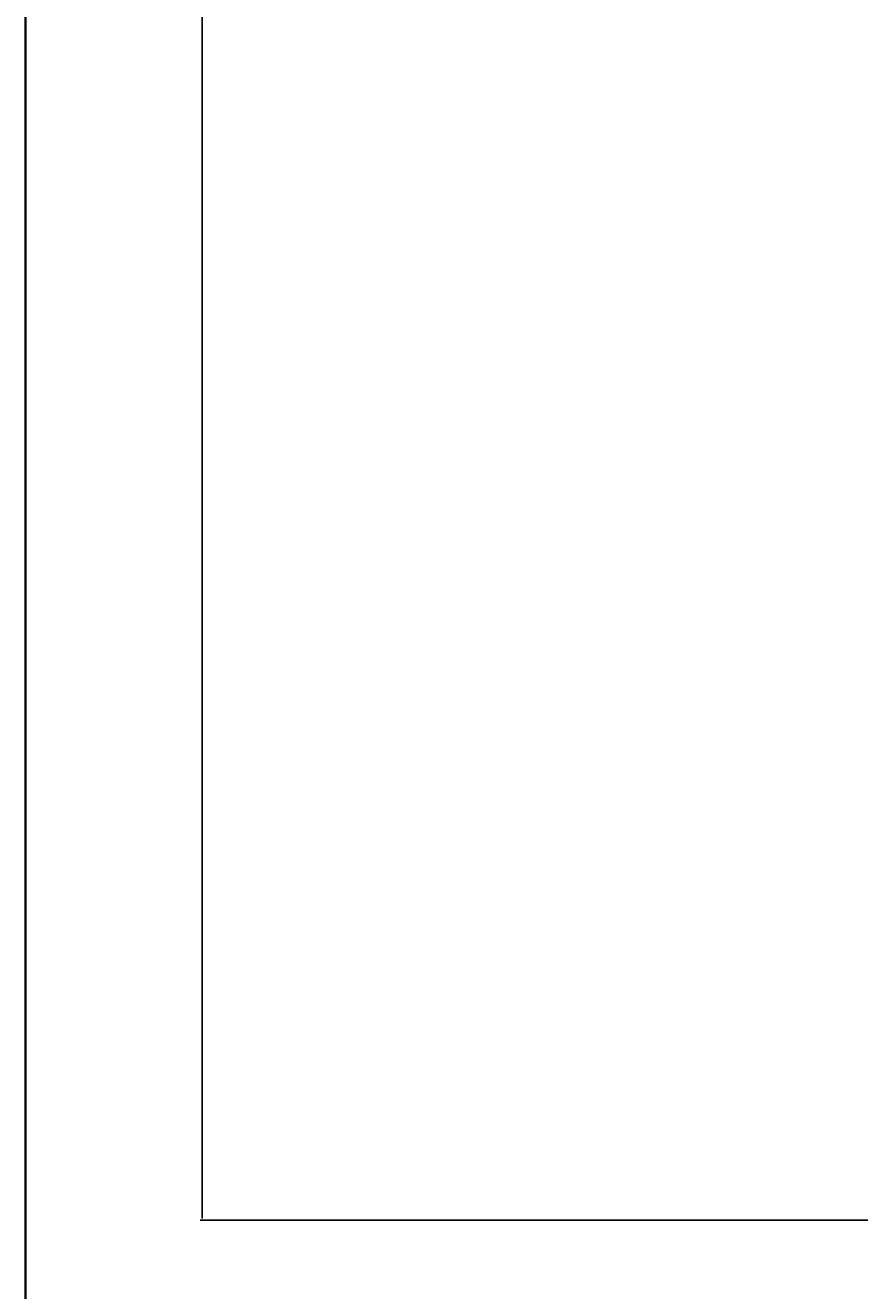
# Model space of a CAD drawing. Units: inches. Extents: x 1885 to 2748, y 783 to 2421.
# Tile 2 of 117: x 1885 to 1969, y 1050 to 1178. Entities that reach past the tile are written whole.
import ezdxf

# ---------------------------------------------------------------- set-up
doc = ezdxf.new("R2010")
doc.units = ezdxf.units.IN
doc.layers.add('A-ANNO-DIMS', color=2, linetype='Continuous', lineweight=18)
doc.layers.add('A-ANNO-TTLB', color=7, linetype='Continuous', lineweight=35)
doc.styles.get("Standard").update_dxf_attribs({"font": 'arial.ttf'})
doc.dimstyles.get("Standard").update_dxf_attribs({"dimtxt": 0.18, "dimasz": 0.18, "dimexe": 0.18, "dimexo": 0.0625, "dimgap": 0.09, "dimtad": 0, "dimtih": 1, "dimtoh": 1, "dimdec": 4, "dimzin": 0, "dimdsep": 46, "dimtxsty": 'Standard', "dimcen": 0.09, "dimadec": 0, "dimazin": 0, "dimtfac": 1, "dimtdec": 4, "dimtofl": 0, "dimtmove": 0, "dimatfit": 3, "dimfxl": 1, "dimtolj": 1, "dimtzin": 0, "dimarcsym": 0})

# ---------------------------------------------------------------- blocks, each defined once
blk = doc.blocks.new('*D45')
at = {"layer": 'A-ANNO-DIMS', "color": 0, "lineweight": -2, "transparency": 16777216}
for p, q in [((1980.71, 1524.01), (1902.84, 1524.01)), ((1903.02, 1523.83), (1903.02, 1290.94)), ((1903.02, 1057.69), (1903.02, 1290.57)), ((1971.21, 1057.51), (1902.84, 1057.51))]:
    blk.add_line(p, q, dxfattribs=at)
at = {"layer": 'A-ANNO-DIMS', "color": 0, "transparency": 16777216}
for points in [[(1902.99, 1523.83), (1903.05, 1523.83), (1903.02, 1524.01)], [(1902.99, 1057.69), (1903.05, 1057.69), (1903.02, 1057.51)]]:
    blk.add_solid(points, dxfattribs=at)
at = {"layer": 'Defpoints', "color": 0, "transparency": 16777216}
for p in [(1903.02, 1524.01), (1980.77, 1524.01), (1971.27, 1057.51)]:
    blk.add_point(p, dxfattribs=at)
at = {"layer": 'A-ANNO-DIMS', "color": 0, "transparency": 16777216, "insert": (1903.02, 1290.76), "char_height": 0.18, "attachment_point": 5}
blk.add_mtext('\\A1;466.5', dxfattribs=at)

msp = doc.modelspace()

# ---------------------------------------------------------------- linework, layer by layer
at = {"layer": 'A-ANNO-TTLB'}
msp.add_lwpolyline([(1885.16, 2409.17), (2748.2, 2409.17), (2748.2, 922.58), (1885.16, 922.58)], close=True, dxfattribs=at)

# ---------------------------------------------------------------- dimensions: what is measured, and where the dimension line sits
at = {"layer": 'A-ANNO-DIMS'}
dim = msp.add_linear_dim(base=(1903.02, 1524.01), p1=(1971.27, 1057.51), p2=(1980.77, 1524.01), angle=90, dimstyle='Standard', override={"dimdec": 1, "dimlfac": 1, "dimrnd": 0, "dimzin": 0, "dimdsep": 46, "dimlunit": 2}, dxfattribs=at)
dim.commit()
dim.dimension.update_dxf_attribs({"geometry": '*D45', "text_midpoint": (1903.02, 1290.76)})

doc.saveas('drawing.dxf')
